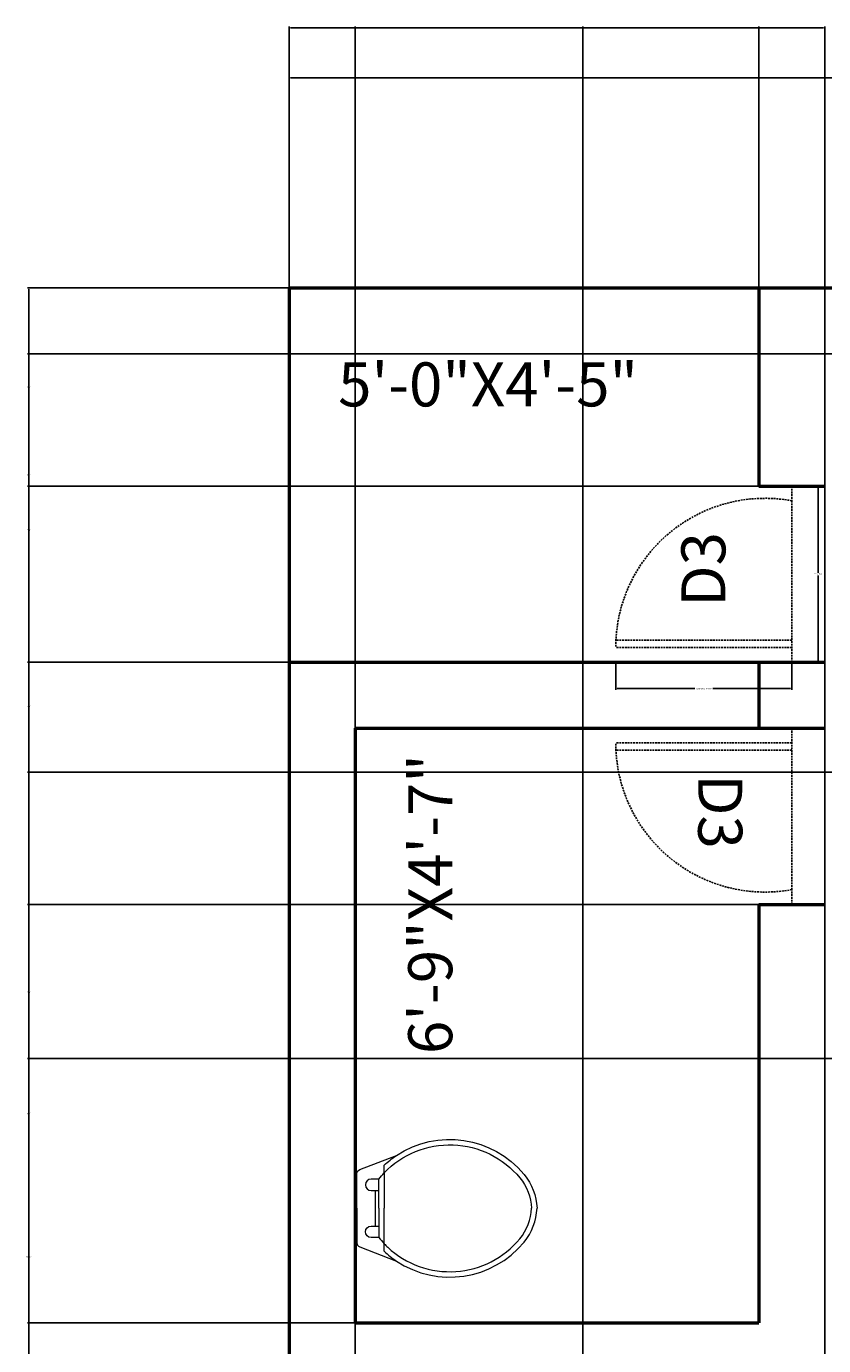
# Model space of a CAD drawing. Units: inches. Extents: x 3 to 576, y -689 to 51.
# Tile 16 of 21: x 3 to 111, y -128 to 51. Entities that reach past the tile are written whole.
import ezdxf

# ---------------------------------------------------------------- set-up
doc = ezdxf.new("R2010")
doc.units = ezdxf.units.IN
doc.header["$MEASUREMENT"] = 0
doc.linetypes.add('DASHED2', pattern=[0.375, 0.25, -0.125])
for name, color, linetype, lineweight in [('A-ANNO-DIMS', 2, 'Continuous', 18), ('A-ANNO-TEXT', 3, 'Continuous', 18), ('A-AREA-IDEN', 7, 'Continuous', 18), ('A-DOOR', 4, 'DASHED2', 25), ('A-FLOR-FIXT', 9, 'Continuous', 18), ('A-WALL', 7, 'Continuous', 50)]:
    doc.layers.add(name, color=color, linetype=linetype, lineweight=lineweight)
doc.styles.get("Standard").update_dxf_attribs({"font": 'arial.ttf'})
doc.dimstyles.get("Standard").update_dxf_attribs({"dimtxt": 0.18, "dimasz": 0.18, "dimexe": 0.18, "dimexo": 0.0625, "dimgap": 0.09, "dimtad": 0, "dimtih": 1, "dimtoh": 1, "dimdec": 0, "dimzin": 0, "dimdsep": 46, "dimlunit": 3, "dimtxsty": 'Standard', "dimcen": 0.09, "dimadec": 0, "dimazin": 0, "dimtfac": 1, "dimtdec": 0, "dimtofl": 0, "dimtmove": 0, "dimatfit": 3, "dimfxl": 1, "dimtolj": 1, "dimtzin": 0, "dimarcsym": 0})

# ---------------------------------------------------------------- blocks, each defined once
blk = doc.blocks.new('*D1')
at = {"layer": 'A-ANNO-DIMS', "color": 0, "lineweight": -2, "transparency": 16777216}
for p, q in [((38.29, 15.75), (38.29, 44.49)), ((38.47, 44.31), (276.45, 44.31)), ((540.11, 44.31), (302.14, 44.31)), ((540.29, 15.75), (540.29, 44.49))]:
    blk.add_line(p, q, dxfattribs=at)
at = {"layer": 'A-ANNO-DIMS', "color": 0, "transparency": 16777216}
for points in [[(38.47, 44.34), (38.47, 44.28), (38.29, 44.31)], [(540.11, 44.34), (540.11, 44.28), (540.29, 44.31)]]:
    blk.add_solid(points, dxfattribs=at)
at = {"layer": 'Defpoints', "color": 0, "transparency": 16777216}
for p in [(540.29, 44.31), (38.29, 15.69), (540.29, 15.69)]:
    blk.add_point(p, dxfattribs=at)
at = {"layer": 'A-ANNO-DIMS', "color": 0, "transparency": 16777216, "insert": (289.29, 44.31), "char_height": 6, "attachment_point": 5}
blk.add_mtext('\\A1;41\'-10"', dxfattribs=at)
blk = doc.blocks.new('WC')
for p, q in [((3.72, 14.21), (3.72, 15.24)), ((3.72, 14.21), (3.72, 9.38)), ((3.72, 4.55), (3.72, 9.38)), ((3.72, 3.52), (3.72, 4.55))]:
    blk.add_line(p, q)
for points in [[(3.72, 14.21, -0.448546), (22.21, 13.53, -0.162618), (23.81, 9.38, -0.470877)], [(5.4, 16.57, -0.383919), (22.78, 13.99, -0.163732), (24.55, 9.38, -0.359733)], [(0, 9.38), (0, 14.07, -0.31031), (0.39, 14.64), (5.4, 16.57, -0.209071)], [(3.72, 15.24, -0.040937), (5.4, 16.57, -0.163732)], [(2.98, 13.36), (1.94, 13.36, 1), (1.94, 11.8), (2.48, 11.8)], [(2.98, 13.36, -0.022712), (3.72, 14.21, -0.162618)], [(2.98, 9.38), (2.98, 13.36, -0.476108)], [(0, 9.38), (0, 4.69, 0.31031), (0.39, 4.12), (5.4, 2.19, 0.209071)], [(2.98, 9.38), (2.98, 5.4, 0.022712)], [(4.22, 4.06, 0.431639), (22.21, 5.23, 0.162618), (23.81, 9.38, 0.470877)], [(5.4, 2.19, 0.383919), (22.78, 4.76, 0.163732), (24.55, 9.38, 0.359733)], [(2.98, 5.4), (1.94, 5.4, -1), (1.94, 6.96), (2.48, 6.96)], [(2.98, 5.4, 0.022712), (3.72, 4.55, 0.162618)], [(3.72, 4.55, 0.014165), (4.22, 4.06, 0.162618)], [(3.72, 3.52, 0.040937), (5.4, 2.19, 0.163732)]]:
    blk.add_lwpolyline(points, format="xyb")
for points in [[(2.48, 11.8), (2.48, 6.96)], [(2.48, 11.8), (2.98, 11.8)], [(2.48, 6.96), (2.98, 6.96)]]:
    blk.add_lwpolyline(points)
blk = doc.blocks.new('DOOR-SWING-750')
for p, q in [((24, 24), (24, 22)), ((24, 22), (24, 2)), ((24, 2), (0, 2)), ((24, 0), (24, 2))]:
    blk.add_line(p, q)
blk.add_arc((20.33, 2), 20.33, 79.6111, 180)
blk = doc.blocks.new('*D13')
at = {"layer": 'A-ANNO-DIMS', "color": 0, "lineweight": -2, "transparency": 16777216}
for p, q in [((82.79, -35.37), (82.79, -39.09)), ((106.79, -35.37), (106.79, -39.09)), ((82.97, -38.91), (93.55, -38.91)), ((106.61, -38.91), (96.04, -38.91))]:
    blk.add_line(p, q, dxfattribs=at)
at = {"layer": 'A-ANNO-DIMS', "color": 0, "transparency": 16777216}
for points in [[(82.97, -38.88), (82.97, -38.94), (82.79, -38.91)], [(106.61, -38.88), (106.61, -38.94), (106.79, -38.91)]]:
    blk.add_solid(points, dxfattribs=at)
at = {"layer": 'Defpoints', "color": 0, "transparency": 16777216}
for p in [(82.79, -35.31), (106.79, -35.31), (106.79, -38.91)]:
    blk.add_point(p, dxfattribs=at)
at = {"layer": 'A-ANNO-DIMS', "color": 0, "transparency": 16777216, "insert": (94.79, -38.91), "char_height": 0.18, "attachment_point": 5}
blk.add_mtext('\\A1;DOOR D3 2\'-0" TYP.', dxfattribs=at)
blk = doc.blocks.new('*D14')
at = {"layer": 'A-ANNO-DIMS', "color": 0, "lineweight": -2, "transparency": 16777216}
for p, q in [((106.86, -11.31), (110.57, -11.31)), ((110.39, -11.49), (110.39, -23.13)), ((110.39, -35.13), (110.39, -23.49)), ((106.86, -35.31), (110.57, -35.31))]:
    blk.add_line(p, q, dxfattribs=at)
at = {"layer": 'A-ANNO-DIMS', "color": 0, "transparency": 16777216}
for points in [[(110.36, -11.49), (110.42, -11.49), (110.39, -11.31)], [(110.36, -35.13), (110.42, -35.13), (110.39, -35.31)]]:
    blk.add_solid(points, dxfattribs=at)
at = {"layer": 'Defpoints', "color": 0, "transparency": 16777216}
for p in [(106.79, -11.31), (110.39, -11.31), (106.79, -35.31)]:
    blk.add_point(p, dxfattribs=at)
at = {"layer": 'A-ANNO-DIMS', "color": 0, "transparency": 16777216, "insert": (110.39, -23.31), "char_height": 0.18, "attachment_point": 5}
blk.add_mtext('\\A1;2\'-0" TYP.', dxfattribs=at)
blk = doc.blocks.new('*D40')
at = {"layer": 'A-ANNO-DIMS', "color": 0, "lineweight": -2, "transparency": 16777216}
for p, q in [((38.29, 15.75), (38.29, 51.32)), ((38.47, 51.14), (69.96, 51.14)), ((102.11, 51.14), (70.62, 51.14)), ((102.29, 15.75), (102.29, 51.32))]:
    blk.add_line(p, q, dxfattribs=at)
at = {"layer": 'A-ANNO-DIMS', "color": 0, "transparency": 16777216}
for points in [[(38.47, 51.17), (38.47, 51.11), (38.29, 51.14)], [(102.11, 51.17), (102.11, 51.11), (102.29, 51.14)]]:
    blk.add_solid(points, dxfattribs=at)
at = {"layer": 'Defpoints', "color": 0, "transparency": 16777216}
for p in [(102.29, 51.14), (38.29, 15.69), (102.29, 15.69)]:
    blk.add_point(p, dxfattribs=at)
at = {"layer": 'A-ANNO-DIMS', "color": 0, "transparency": 16777216, "insert": (70.29, 51.14), "char_height": 0.18, "attachment_point": 5}
blk.add_mtext('\\A1;5\'-4"', dxfattribs=at)
blk = doc.blocks.new('*D41')
at = {"layer": 'A-ANNO-DIMS', "color": 0, "lineweight": -2, "transparency": 16777216}
for p, q in [((102.29, 15.75), (102.29, 51.32)), ((102.47, 51.14), (106.46, 51.14)), ((111.11, 51.14), (107.12, 51.14)), ((111.29, 6.75), (111.29, 51.32))]:
    blk.add_line(p, q, dxfattribs=at)
at = {"layer": 'A-ANNO-DIMS', "color": 0, "transparency": 16777216}
for points in [[(102.47, 51.17), (102.47, 51.11), (102.29, 51.14)], [(111.11, 51.17), (111.11, 51.11), (111.29, 51.14)]]:
    blk.add_solid(points, dxfattribs=at)
at = {"layer": 'Defpoints', "color": 0, "transparency": 16777216}
for p in [(111.29, 51.14), (102.29, 15.69), (111.29, 6.69)]:
    blk.add_point(p, dxfattribs=at)
at = {"layer": 'A-ANNO-DIMS', "color": 0, "transparency": 16777216, "insert": (106.79, 51.14), "char_height": 0.18, "attachment_point": 5}
blk.add_mtext('\\A1;0\'-9"', dxfattribs=at)
blk = doc.blocks.new('*D53')
at = {"layer": 'A-ANNO-DIMS', "color": 0, "lineweight": -2, "transparency": 16777216}
for p, q in [((38.23, 15.69), (2.66, 15.69)), ((2.84, 15.51), (2.84, -9.63)), ((2.84, -35.13), (2.84, -9.99)), ((38.23, -35.31), (2.66, -35.31))]:
    blk.add_line(p, q, dxfattribs=at)
at = {"layer": 'A-ANNO-DIMS', "color": 0, "transparency": 16777216}
for points in [[(2.81, 15.51), (2.87, 15.51), (2.84, 15.69)], [(2.81, -35.13), (2.87, -35.13), (2.84, -35.31)]]:
    blk.add_solid(points, dxfattribs=at)
at = {"layer": 'Defpoints', "color": 0, "transparency": 16777216}
for p in [(38.29, 15.69), (2.84, -35.31), (38.29, -35.31)]:
    blk.add_point(p, dxfattribs=at)
at = {"layer": 'A-ANNO-DIMS', "color": 0, "transparency": 16777216, "insert": (2.84, -9.81), "char_height": 0.18, "attachment_point": 5}
blk.add_mtext('\\A1;4\'-3"', dxfattribs=at)
blk = doc.blocks.new('*D54')
at = {"layer": 'A-ANNO-DIMS', "color": 0, "lineweight": -2, "transparency": 16777216}
for p, q in [((38.23, -35.31), (2.66, -35.31)), ((2.84, -35.49), (2.84, -80.13)), ((2.84, -125.13), (2.84, -80.49)), ((47.23, -125.31), (2.66, -125.31))]:
    blk.add_line(p, q, dxfattribs=at)
at = {"layer": 'A-ANNO-DIMS', "color": 0, "transparency": 16777216}
for points in [[(2.81, -35.49), (2.87, -35.49), (2.84, -35.31)], [(2.81, -125.13), (2.87, -125.13), (2.84, -125.31)]]:
    blk.add_solid(points, dxfattribs=at)
at = {"layer": 'Defpoints', "color": 0, "transparency": 16777216}
for p in [(38.29, -35.31), (2.84, -125.31), (47.29, -125.31)]:
    blk.add_point(p, dxfattribs=at)
at = {"layer": 'A-ANNO-DIMS', "color": 0, "transparency": 16777216, "insert": (2.84, -80.31), "char_height": 0.18, "attachment_point": 5}
blk.add_mtext('\\A1;7\'-6"', dxfattribs=at)
blk = doc.blocks.new('*D55')
at = {"layer": 'A-ANNO-DIMS', "color": 0, "lineweight": -2, "transparency": 16777216}
for p, q in [((47.23, -125.31), (2.66, -125.31)), ((2.84, -125.49), (2.84, -129.63)), ((2.84, -134.13), (2.84, -129.99)), ((38.23, -134.31), (2.66, -134.31))]:
    blk.add_line(p, q, dxfattribs=at)
at = {"layer": 'A-ANNO-DIMS', "color": 0, "transparency": 16777216}
for points in [[(2.81, -125.49), (2.87, -125.49), (2.84, -125.31)], [(2.81, -134.13), (2.87, -134.13), (2.84, -134.31)]]:
    blk.add_solid(points, dxfattribs=at)
at = {"layer": 'Defpoints', "color": 0, "transparency": 16777216}
for p in [(47.29, -125.31), (2.84, -134.31), (38.29, -134.31)]:
    blk.add_point(p, dxfattribs=at)
at = {"layer": 'A-ANNO-DIMS', "color": 0, "transparency": 16777216, "insert": (2.84, -129.81), "char_height": 0.18, "attachment_point": 5}
blk.add_mtext('\\A1;0\'-9"', dxfattribs=at)
blk = doc.blocks.new('*D64')
at = {"layer": 'A-ANNO-DIMS', "color": 0, "lineweight": -2, "transparency": 16777216}
for p, q in [((540.23, 15.69), (2.66, 15.69)), ((2.84, 15.51), (2.84, -17.13)), ((2.84, -50.13), (2.84, -17.49)), ((531.23, -50.31), (2.66, -50.31))]:
    blk.add_line(p, q, dxfattribs=at)
at = {"layer": 'A-ANNO-DIMS', "color": 0, "transparency": 16777216}
for points in [[(2.81, 15.51), (2.87, 15.51), (2.84, 15.69)], [(2.81, -50.13), (2.87, -50.13), (2.84, -50.31)]]:
    blk.add_solid(points, dxfattribs=at)
at = {"layer": 'Defpoints', "color": 0, "transparency": 16777216}
for p in [(540.29, 15.69), (2.84, -50.31), (531.29, -50.31)]:
    blk.add_point(p, dxfattribs=at)
at = {"layer": 'A-ANNO-DIMS', "color": 0, "transparency": 16777216, "insert": (2.84, -17.31), "char_height": 0.18, "attachment_point": 5}
blk.add_mtext('\\A1;5\'-6"', dxfattribs=at)
blk = doc.blocks.new('*D65')
at = {"layer": 'A-ANNO-DIMS', "color": 0, "lineweight": -2, "transparency": 16777216}
for p, q in [((531.23, -50.31), (2.66, -50.31)), ((2.84, -50.49), (2.84, -116.13)), ((2.84, -182.13), (2.84, -116.49)), ((531.23, -182.31), (2.66, -182.31))]:
    blk.add_line(p, q, dxfattribs=at)
at = {"layer": 'A-ANNO-DIMS', "color": 0, "transparency": 16777216}
for points in [[(2.81, -50.49), (2.87, -50.49), (2.84, -50.31)], [(2.81, -182.13), (2.87, -182.13), (2.84, -182.31)]]:
    blk.add_solid(points, dxfattribs=at)
at = {"layer": 'Defpoints', "color": 0, "transparency": 16777216}
for p in [(531.29, -50.31), (2.84, -182.31), (531.29, -182.31)]:
    blk.add_point(p, dxfattribs=at)
at = {"layer": 'A-ANNO-DIMS', "color": 0, "transparency": 16777216, "insert": (2.84, -116.31), "char_height": 0.18, "attachment_point": 5}
blk.add_mtext('\\A1;11\'-0"', dxfattribs=at)
blk = doc.blocks.new('*D98')
at = {"layer": 'A-ANNO-DIMS', "color": 0, "lineweight": -2, "transparency": 16777216}
for p, q in [((102.23, 15.69), (2.66, 15.69)), ((2.84, 15.51), (2.84, 2.37)), ((2.84, -11.13), (2.84, 2.01)), ((102.23, -11.31), (2.66, -11.31))]:
    blk.add_line(p, q, dxfattribs=at)
at = {"layer": 'A-ANNO-DIMS', "color": 0, "transparency": 16777216}
for points in [[(2.81, 15.51), (2.87, 15.51), (2.84, 15.69)], [(2.81, -11.13), (2.87, -11.13), (2.84, -11.31)]]:
    blk.add_solid(points, dxfattribs=at)
at = {"layer": 'Defpoints', "color": 0, "transparency": 16777216}
for p in [(102.29, 15.69), (2.84, -11.31), (102.29, -11.31)]:
    blk.add_point(p, dxfattribs=at)
at = {"layer": 'A-ANNO-DIMS', "color": 0, "transparency": 16777216, "insert": (2.84, 2.19), "char_height": 0.18, "attachment_point": 5}
blk.add_mtext('\\A1;2\'-3"', dxfattribs=at)
blk = doc.blocks.new('*D99')
at = {"layer": 'A-ANNO-DIMS', "color": 0, "lineweight": -2, "transparency": 16777216}
for p, q in [((102.23, -68.31), (2.66, -68.31)), ((2.84, -68.49), (2.84, -96.63)), ((2.84, -125.13), (2.84, -96.99)), ((102.23, -125.31), (2.66, -125.31))]:
    blk.add_line(p, q, dxfattribs=at)
at = {"layer": 'A-ANNO-DIMS', "color": 0, "transparency": 16777216}
for points in [[(2.81, -68.49), (2.87, -68.49), (2.84, -68.31)], [(2.81, -125.13), (2.87, -125.13), (2.84, -125.31)]]:
    blk.add_solid(points, dxfattribs=at)
at = {"layer": 'Defpoints', "color": 0, "transparency": 16777216}
for p in [(102.29, -68.31), (2.84, -125.31), (102.29, -125.31)]:
    blk.add_point(p, dxfattribs=at)
at = {"layer": 'A-ANNO-DIMS', "color": 0, "transparency": 16777216, "insert": (2.84, -96.81), "char_height": 0.18, "attachment_point": 5}
blk.add_mtext('\\A1;4\'-9"', dxfattribs=at)
blk = doc.blocks.new('*D100')
at = {"layer": 'A-ANNO-DIMS', "color": 0, "lineweight": -2, "transparency": 16777216}
for p, q in [((255.23, 6.69), (2.66, 6.69)), ((2.84, 6.51), (2.84, -41.13)), ((2.84, -89.13), (2.84, -41.49)), ((255.23, -89.31), (2.66, -89.31))]:
    blk.add_line(p, q, dxfattribs=at)
at = {"layer": 'A-ANNO-DIMS', "color": 0, "transparency": 16777216}
for points in [[(2.81, 6.51), (2.87, 6.51), (2.84, 6.69)], [(2.81, -89.13), (2.87, -89.13), (2.84, -89.31)]]:
    blk.add_solid(points, dxfattribs=at)
at = {"layer": 'Defpoints', "color": 0, "transparency": 16777216}
for p in [(255.29, 6.69), (2.84, -89.31), (255.29, -89.31)]:
    blk.add_point(p, dxfattribs=at)
at = {"layer": 'A-ANNO-DIMS', "color": 0, "transparency": 16777216, "insert": (2.84, -41.31), "char_height": 0.18, "attachment_point": 5}
blk.add_mtext('\\A1;8\'-0"', dxfattribs=at)
blk = doc.blocks.new('*D101')
at = {"layer": 'A-ANNO-DIMS', "color": 0, "lineweight": -2, "transparency": 16777216}
for p, q in [((47.29, -254.25), (47.29, 51.32)), ((47.47, 51.14), (62.46, 51.14)), ((78.11, 51.14), (63.12, 51.14)), ((78.29, -254.25), (78.29, 51.32))]:
    blk.add_line(p, q, dxfattribs=at)
at = {"layer": 'A-ANNO-DIMS', "color": 0, "transparency": 16777216}
for points in [[(47.47, 51.17), (47.47, 51.11), (47.29, 51.14)], [(78.11, 51.17), (78.11, 51.11), (78.29, 51.14)]]:
    blk.add_solid(points, dxfattribs=at)
at = {"layer": 'Defpoints', "color": 0, "transparency": 16777216}
for p in [(78.29, 51.14), (47.29, -254.31), (78.29, -254.31)]:
    blk.add_point(p, dxfattribs=at)
at = {"layer": 'A-ANNO-DIMS', "color": 0, "transparency": 16777216, "insert": (62.79, 51.14), "char_height": 0.18, "attachment_point": 5}
blk.add_mtext('\\A1;2\'-7"', dxfattribs=at)
blk = doc.blocks.new('*D119')
at = {"layer": 'A-ANNO-DIMS', "color": 0, "lineweight": -2, "transparency": 16777216}
for p, q in [((47.29, -311.25), (47.29, 51.32)), ((47.47, 51.14), (78.96, 51.14)), ((111.11, 51.14), (79.62, 51.14)), ((111.29, -311.25), (111.29, 51.32))]:
    blk.add_line(p, q, dxfattribs=at)
at = {"layer": 'A-ANNO-DIMS', "color": 0, "transparency": 16777216}
for points in [[(47.47, 51.17), (47.47, 51.11), (47.29, 51.14)], [(111.11, 51.17), (111.11, 51.11), (111.29, 51.14)]]:
    blk.add_solid(points, dxfattribs=at)
at = {"layer": 'Defpoints', "color": 0, "transparency": 16777216}
for p in [(111.29, 51.14), (47.29, -311.31), (111.29, -311.31)]:
    blk.add_point(p, dxfattribs=at)
at = {"layer": 'A-ANNO-DIMS', "color": 0, "transparency": 16777216, "insert": (79.29, 51.14), "char_height": 0.18, "attachment_point": 5}
blk.add_mtext('\\A1;5\'-4"', dxfattribs=at)

msp = doc.modelspace()

# ---------------------------------------------------------------- linework, layer by layer
at = {"layer": 'A-DOOR'}
for p, q in [((106.79, -32.31), (82.79, -32.31)), ((106.79, -47.31), (82.79, -47.31))]:
    msp.add_line(p, q, dxfattribs=at)
at = {"layer": 'A-WALL'}
for p, q in [((38.29, 15.69), (38.29, -653.31)), ((38.29, 15.69), (540.29, 15.69)), ((102.29, 15.69), (102.29, -11.31)), ((102.29, -11.31), (111.29, -11.31)), ((38.29, -35.31), (102.29, -35.31)), ((102.29, -35.31), (111.29, -35.31)), ((102.29, -35.31), (102.29, -44.31)), ((47.29, -44.31), (47.29, -125.31)), ((47.29, -44.31), (102.29, -44.31)), ((102.29, -44.31), (111.29, -44.31)), ((102.29, -68.31), (111.29, -68.31)), ((102.29, -68.31), (102.29, -125.31)), ((47.29, -125.31), (102.29, -125.31))]:
    msp.add_line(p, q, dxfattribs=at)

# ---------------------------------------------------------------- block references
at = {"layer": 'A-DOOR'}
msp.add_blockref('DOOR-SWING-750', (82.79, -35.31), dxfattribs=at)
at = {"layer": 'A-DOOR', "extrusion": (0, 0, -1), "zscale": -1, "rotation": 180}
msp.add_blockref('DOOR-SWING-750', (-82.79, -44.31), dxfattribs=at)
at = {"layer": 'A-FLOR-FIXT'}
msp.add_blockref('WC', (47.52, -119.1), dxfattribs=at)

# ---------------------------------------------------------------- texts
at = {"layer": 'A-ANNO-TEXT', "char_height": 6, "attachment_point": 1}
for insert, rotation in [((91.73, -27.76), 90), ((100.03, -50.57), 270)]:
    msp.add_mtext('D3', dxfattribs=dict(at, insert=insert, rotation=rotation))
at = {"layer": 'A-AREA-IDEN', "insert": (44.97, 5.54), "char_height": 6, "attachment_point": 1}
msp.add_mtext('5\'-0"X4\'-5"', dxfattribs=at)
at = {"layer": 'A-AREA-IDEN', "insert": (54.52, -88.71), "char_height": 6, "attachment_point": 1, "rotation": 90}
msp.add_mtext('6\'-9"X4\'-7"', dxfattribs=at)

# ---------------------------------------------------------------- dimensions: what is measured, and where the dimension line sits
at = {"layer": 'A-ANNO-DIMS'}
for base, p1, p2, override, picture, middle in [((102.29, 51.14), (38.29, 15.69), (102.29, 15.69), {"dimdec": 1, "dimlfac": 1, "dimrnd": 0, "dimzin": 1, "dimdsep": 46, "dimlunit": 4, "dimfrac": 2}, '*D40', (70.29, 51.14)), ((78.29, 51.14), (47.29, -254.31), (78.29, -254.31), {"dimdec": 1, "dimlfac": 1, "dimrnd": 0, "dimzin": 1, "dimdsep": 46, "dimlunit": 4, "dimfrac": 2}, '*D101', (62.79, 51.14)), ((111.29, 51.14), (47.29, -311.31), (111.29, -311.31), {"dimdec": 1, "dimlfac": 1, "dimrnd": 0, "dimzin": 1, "dimdsep": 46, "dimlunit": 4, "dimfrac": 2}, '*D119', (79.29, 51.14)), ((111.29, 51.14), (102.29, 15.69), (111.29, 6.69), {"dimdec": 1, "dimlfac": 1, "dimrnd": 0, "dimzin": 1, "dimdsep": 46, "dimlunit": 4, "dimfrac": 2}, '*D41', (106.79, 51.14)), ((540.29, 44.31), (38.29, 15.69), (540.29, 15.69), {"dimtxt": 6, "dimclrd": 0, "dimclre": 0, "dimclrt": 0}, '*D1', (289.29, 44.31))]:
    dim = msp.add_linear_dim(base=base, p1=p1, p2=p2, dimstyle='Standard', override=override, dxfattribs=at)
    dim.commit()
    dim.dimension.update_dxf_attribs({"geometry": picture, "text_midpoint": middle})
for base, p1, p2, picture, middle in [((2.84, -35.31), (38.29, 15.69), (38.29, -35.31), '*D53', (2.84, -9.81)), ((2.84, -50.31), (540.29, 15.69), (531.29, -50.31), '*D64', (2.84, -17.31)), ((2.84, -11.31), (102.29, 15.69), (102.29, -11.31), '*D98', (2.84, 2.19)), ((2.84, -89.31), (255.29, 6.69), (255.29, -89.31), '*D100', (2.84, -41.31)), ((2.84, -125.31), (38.29, -35.31), (47.29, -125.31), '*D54', (2.84, -80.31)), ((2.84, -182.31), (531.29, -50.31), (531.29, -182.31), '*D65', (2.84, -116.31)), ((2.84, -125.31), (102.29, -68.31), (102.29, -125.31), '*D99', (2.84, -96.81)), ((2.84, -134.31), (47.29, -125.31), (38.29, -134.31), '*D55', (2.84, -129.81))]:
    dim = msp.add_linear_dim(base=base, p1=p1, p2=p2, angle=90, dimstyle='Standard', override={"dimdec": 1, "dimlfac": 1, "dimrnd": 0, "dimzin": 1, "dimdsep": 46, "dimlunit": 4, "dimfrac": 2}, dxfattribs=at)
    dim.commit()
    dim.dimension.update_dxf_attribs({"geometry": picture, "text_midpoint": middle})
dim = msp.add_linear_dim(base=(110.39, -11.31), p1=(106.79, -35.31), p2=(106.79, -11.31), angle=90, text='<> TYP.', dimstyle='Standard', override={"dimdec": 1, "dimlfac": 1, "dimrnd": 0, "dimzin": 1, "dimdsep": 46, "dimlunit": 4, "dimfrac": 2}, dxfattribs=at)
dim.commit()
dim.dimension.update_dxf_attribs({"geometry": '*D14', "text_midpoint": (110.39, -23.31)})
dim = msp.add_linear_dim(base=(106.79, -38.91), p1=(82.79, -35.31), p2=(106.79, -35.31), text='DOOR D3 <> TYP.', dimstyle='Standard', override={"dimdec": 1, "dimlfac": 1, "dimrnd": 0, "dimzin": 1, "dimdsep": 46, "dimlunit": 4, "dimfrac": 2}, dxfattribs=at)
dim.commit()
dim.dimension.update_dxf_attribs({"geometry": '*D13', "text_midpoint": (94.79, -38.91)})

doc.saveas('drawing.dxf')
